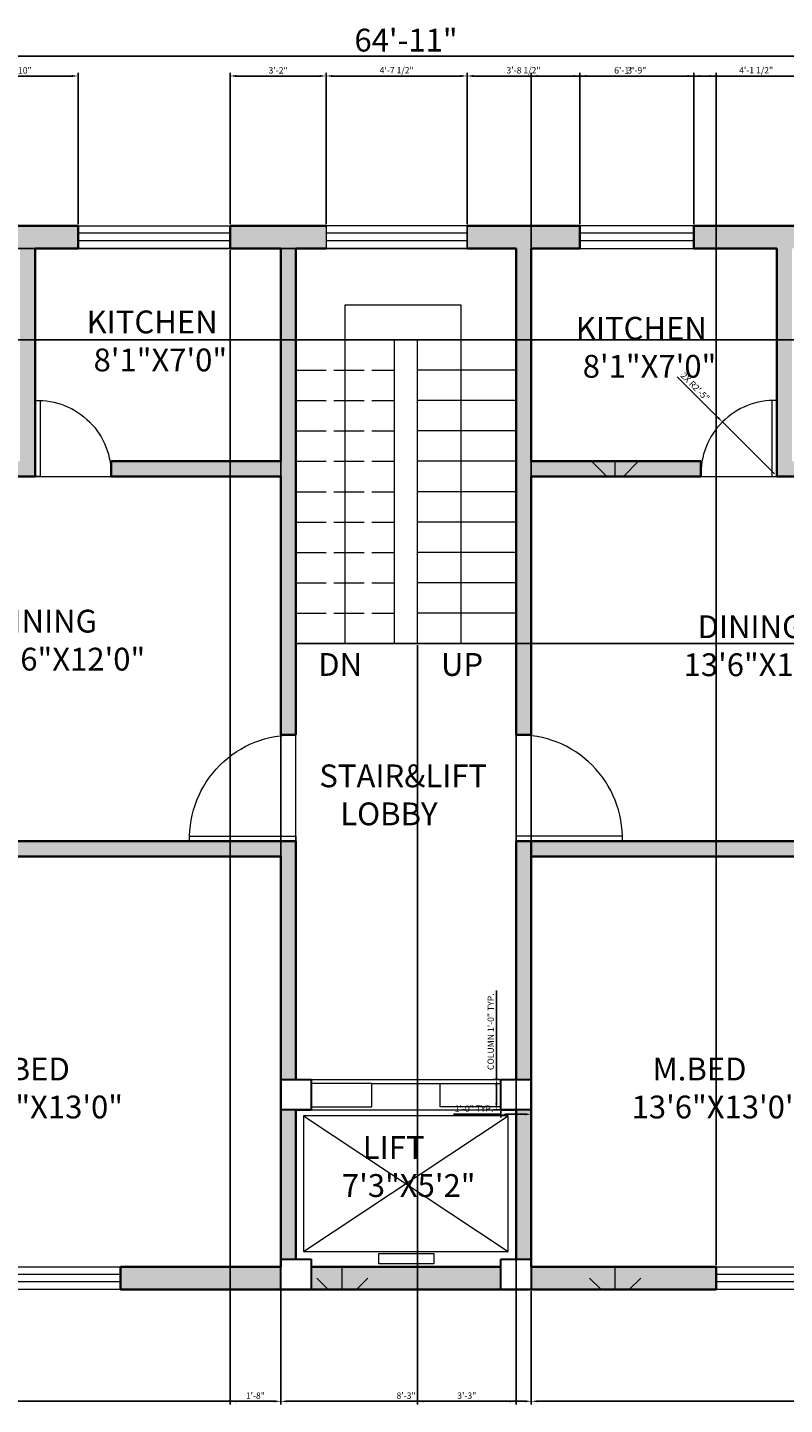
# Model space of a CAD drawing. Units: inches. Extents: x 1851 to 3979, y 3948 to 8145.
# Tile 3 of 4: x 2139 to 2438, y 3948 to 4491. Entities that reach past the tile are written whole.
import ezdxf

# ---------------------------------------------------------------- set-up
doc = ezdxf.new("R2010")
doc.units = ezdxf.units.IN
doc.linetypes.add('ACAD_ISO02W100', pattern=[15, 12, -3])
for name, color, linetype, lineweight in [('A-ANNO-DIMS', 2, 'Continuous', 18), ('A-ANNO-TEXT', 7, 'Continuous', 18), ('A-GLAZ', 140, 'Continuous', 18), ('A-WALL', 7, 'Continuous', 35)]:
    doc.layers.add(name, color=color, linetype=linetype, lineweight=lineweight)
for name, color, linetype, lineweight, true_color in [('A-AREA-IDEN', 9, 'Continuous', 18, 0xc7c8ca), ('A-COLS', 240, 'Continuous', 30, 0xed1f24), ('A-COLS-PATT', 251, 'Continuous', 13, 0x636466), ('A-DOOR', 52, 'Continuous', 18, 0xc8c92d), ('A-FLOR-EVTR', 242, 'Continuous', 18, 0xcd2027), ('A-FLOR-STRS', 242, 'Continuous', 18, 0xcd2027), ('A-FLOR-STRS-OVHD', 242, 'ACAD_ISO02W100', 13, 0xcd2027), ('A-WALL-PATT', 159, 'Continuous', 13, 0x22346e)]:
    doc.layers.add(name, color=color, linetype=linetype, lineweight=lineweight, true_color=true_color)
doc.styles.get("Standard").update_dxf_attribs({"font": 'arial.ttf'})
doc.dimstyles.new('ISO-25', dxfattribs={"dimtxt": 2.5, "dimasz": 2.5, "dimexe": 1.25, "dimexo": 0.625, "dimtad": 1, "dimlunit": 3, "dimtxsty": 'Standard', "dimcen": 2.5, "dimadec": 0, "dimazin": 0, "dimtfac": 1, "dimtmove": 0, "dimatfit": 3, "dimfxl": 1, "dimarcsym": 0})

# ---------------------------------------------------------------- blocks, each defined once
blk = doc.blocks.new('*D1')
at = {"layer": 'A-ANNO-DIMS', "color": 0, "lineweight": -2, "transparency": 16777216}
for p, q in [((1898.74, 4438.02), (1898.74, 4480.98)), ((1901.24, 4479.73), (2675.24, 4479.73)), ((2677.74, 4438.02), (2677.74, 4480.98))]:
    blk.add_line(p, q, dxfattribs=at)
at = {"layer": 'A-ANNO-DIMS', "color": 0, "transparency": 16777216}
for points in [[(1901.24, 4480.15), (1901.24, 4479.31), (1898.74, 4479.73)], [(2675.24, 4480.15), (2675.24, 4479.31), (2677.74, 4479.73)]]:
    blk.add_solid(points, dxfattribs=at)
at = {"layer": 'Defpoints', "color": 0, "transparency": 16777216}
for p in [(2677.74, 4479.73), (1898.74, 4437.39), (2677.74, 4437.39)]:
    blk.add_point(p, dxfattribs=at)
at = {"layer": 'A-ANNO-DIMS', "color": 0, "transparency": 16777216, "insert": (2288.24, 4484.95), "char_height": 9, "attachment_point": 5}
blk.add_mtext('64\'-11"', dxfattribs=at)
blk = doc.blocks.new('DOOR-SINGLE-42IN')
for p, q in [((42, 42), (40, 42)), ((40, 42), (40, 0)), ((42, 0), (42, 42)), ((40, 0), (42, 0))]:
    blk.add_line(p, q)
blk.add_arc((41, 1), 41.01, 88.6028, 181.3972)
blk = doc.blocks.new('DOOR-SINGLE-30IN')
for p, q in [((30, 2), (0, 2)), ((0, 2), (0, 0)), ((0, 0), (30, 0)), ((30, 0), (30, 2))]:
    blk.add_line(p, q)
blk.add_arc((1, 1), 29.02, 358.0251, 91.9749)
blk = doc.blocks.new('WINDOW-60IN')
for p, q in [((0, 9), (60, 9)), ((0, 0), (0, 9)), ((0, 6), (60, 6)), ((60, 9), (60, 0)), ((0, 3), (60, 3)), ((60, 0), (0, 0))]:
    blk.add_line(p, q)
blk = doc.blocks.new('COLUMN-12X12IN')
for p, q in [((0, 0), (0, 12)), ((0, 12), (12, 12)), ((12, 12), (12, 0)), ((12, 0), (0, 0))]:
    blk.add_line(p, q)
blk = doc.blocks.new('*D16')
at = {"layer": 'A-ANNO-DIMS', "color": 0, "lineweight": -2, "transparency": 16777216}
for p, q in [((2323.94, 4075.85), (2323.94, 4110.92)), ((2325.11, 4075.85), (2322.69, 4075.85)), ((2323.94, 4066.35), (2323.94, 4073.35)), ((2325.11, 4063.85), (2322.69, 4063.85))]:
    blk.add_line(p, q, dxfattribs=at)
at = {"layer": 'A-ANNO-DIMS', "color": 0, "transparency": 16777216}
for points in [[(2323.52, 4073.35), (2324.35, 4073.35), (2323.94, 4075.85)], [(2323.52, 4066.35), (2324.35, 4066.35), (2323.94, 4063.85)]]:
    blk.add_solid(points, dxfattribs=at)
at = {"layer": 'Defpoints', "color": 0, "transparency": 16777216}
for p in [(2323.94, 4075.85), (2325.74, 4075.85), (2325.74, 4063.85)]:
    blk.add_point(p, dxfattribs=at)
at = {"layer": 'A-ANNO-DIMS', "color": 0, "transparency": 16777216, "insert": (2322.02, 4094.64), "char_height": 2.5, "attachment_point": 5, "rotation": 90}
blk.add_mtext('COLUMN 1\'-0" TYP.', dxfattribs=at)
blk = doc.blocks.new('*D17')
at = {"layer": 'A-ANNO-DIMS', "color": 0, "lineweight": -2, "transparency": 16777216}
for p, q in [((2325.74, 4062.05), (2306.98, 4062.05)), ((2325.74, 4063.23), (2325.74, 4060.8)), ((2335.24, 4062.05), (2328.24, 4062.05)), ((2337.74, 4063.23), (2337.74, 4060.8))]:
    blk.add_line(p, q, dxfattribs=at)
at = {"layer": 'A-ANNO-DIMS', "color": 0, "transparency": 16777216}
for points in [[(2328.24, 4062.47), (2328.24, 4061.64), (2325.74, 4062.05)], [(2335.24, 4062.47), (2335.24, 4061.64), (2337.74, 4062.05)]]:
    blk.add_solid(points, dxfattribs=at)
at = {"layer": 'Defpoints', "color": 0, "transparency": 16777216}
for p in [(2325.74, 4063.85), (2325.74, 4062.05), (2337.74, 4063.85)]:
    blk.add_point(p, dxfattribs=at)
at = {"layer": 'A-ANNO-DIMS', "color": 0, "transparency": 16777216, "insert": (2315.11, 4063.96), "char_height": 2.5, "attachment_point": 5}
blk.add_mtext('1\'-0" TYP.', dxfattribs=at)
blk = doc.blocks.new('*D24')
at = {"layer": 'A-ANNO-DIMS', "color": 0, "lineweight": -2, "transparency": 16777216}
for p, q in [((1898.74, 3992.23), (1898.74, 3947.5)), ((2238.74, 3992.23), (2238.74, 3947.5)), ((1901.24, 3948.75), (2236.24, 3948.75))]:
    blk.add_line(p, q, dxfattribs=at)
at = {"layer": 'A-ANNO-DIMS', "color": 0, "transparency": 16777216}
for points in [[(1901.24, 3949.17), (1901.24, 3948.34), (1898.74, 3948.75)], [(2236.24, 3949.17), (2236.24, 3948.34), (2238.74, 3948.75)]]:
    blk.add_solid(points, dxfattribs=at)
at = {"layer": 'Defpoints', "color": 0, "transparency": 16777216}
for p in [(1898.74, 3992.85), (2238.74, 3992.85), (2238.74, 3948.75)]:
    blk.add_point(p, dxfattribs=at)
at = {"layer": 'A-ANNO-DIMS', "color": 0, "transparency": 16777216, "insert": (2068.74, 3950.66), "char_height": 2.5, "attachment_point": 5}
blk.add_mtext('28\'-4"', dxfattribs=at)
blk = doc.blocks.new('*D25')
at = {"layer": 'A-ANNO-DIMS', "color": 0, "lineweight": -2, "transparency": 16777216}
for p, q in [((2238.74, 3992.23), (2238.74, 3947.5)), ((2337.74, 3992.23), (2337.74, 3947.5)), ((2241.24, 3948.75), (2335.24, 3948.75))]:
    blk.add_line(p, q, dxfattribs=at)
at = {"layer": 'A-ANNO-DIMS', "color": 0, "transparency": 16777216}
for points in [[(2241.24, 3949.17), (2241.24, 3948.34), (2238.74, 3948.75)], [(2335.24, 3949.17), (2335.24, 3948.34), (2337.74, 3948.75)]]:
    blk.add_solid(points, dxfattribs=at)
at = {"layer": 'Defpoints', "color": 0, "transparency": 16777216}
for p in [(2238.74, 3992.85), (2337.74, 3992.85), (2337.74, 3948.75)]:
    blk.add_point(p, dxfattribs=at)
at = {"layer": 'A-ANNO-DIMS', "color": 0, "transparency": 16777216, "insert": (2288.24, 3950.66), "char_height": 2.5, "attachment_point": 5}
blk.add_mtext('8\'-3"', dxfattribs=at)
blk = doc.blocks.new('*D26')
at = {"layer": 'A-ANNO-DIMS', "color": 0, "lineweight": -2, "transparency": 16777216}
for p, q in [((2337.74, 3992.23), (2337.74, 3947.5)), ((2677.74, 3992.23), (2677.74, 3947.5)), ((2340.24, 3948.75), (2675.24, 3948.75))]:
    blk.add_line(p, q, dxfattribs=at)
at = {"layer": 'A-ANNO-DIMS', "color": 0, "transparency": 16777216}
for points in [[(2340.24, 3949.17), (2340.24, 3948.34), (2337.74, 3948.75)], [(2675.24, 3949.17), (2675.24, 3948.34), (2677.74, 3948.75)]]:
    blk.add_solid(points, dxfattribs=at)
at = {"layer": 'Defpoints', "color": 0, "transparency": 16777216}
for p in [(2337.74, 3992.85), (2677.74, 3992.85), (2677.74, 3948.75)]:
    blk.add_point(p, dxfattribs=at)
at = {"layer": 'A-ANNO-DIMS', "color": 0, "transparency": 16777216, "insert": (2507.74, 3950.66), "char_height": 2.5, "attachment_point": 5}
blk.add_mtext('28\'-4"', dxfattribs=at)
blk = doc.blocks.new('*D29')
at = {"layer": 'A-ANNO-DIMS', "color": 0, "lineweight": -2, "transparency": 16777216}
for p, q in [((2337.74, 4002.48), (2337.74, 4473.2)), ((2340.24, 4471.95), (2408.24, 4471.95)), ((2410.74, 4002.48), (2410.74, 4473.2))]:
    blk.add_line(p, q, dxfattribs=at)
at = {"layer": 'A-ANNO-DIMS', "color": 0, "transparency": 16777216}
for points in [[(2340.24, 4472.37), (2340.24, 4471.54), (2337.74, 4471.95)], [(2408.24, 4472.37), (2408.24, 4471.54), (2410.74, 4471.95)]]:
    blk.add_solid(points, dxfattribs=at)
at = {"layer": 'Defpoints', "color": 0, "transparency": 16777216}
for p in [(2410.74, 4471.95), (2337.74, 4001.85), (2410.74, 4001.85)]:
    blk.add_point(p, dxfattribs=at)
at = {"layer": 'A-ANNO-DIMS', "color": 0, "transparency": 16777216, "insert": (2374.24, 4473.86), "char_height": 2.5, "attachment_point": 5}
blk.add_mtext('6\'-1"', dxfattribs=at)
blk = doc.blocks.new('*D33')
at = {"layer": 'A-ANNO-DIMS', "color": 0, "lineweight": -2, "transparency": 16777216}
for p, q in [((2245.36, 4367.85), (2723.09, 4367.85)), ((2721.84, 4250.35), (2721.84, 4365.35)), ((2245.36, 4247.85), (2723.09, 4247.85))]:
    blk.add_line(p, q, dxfattribs=at)
at = {"layer": 'A-ANNO-DIMS', "color": 0, "transparency": 16777216}
for points in [[(2721.42, 4365.35), (2722.25, 4365.35), (2721.84, 4367.85)], [(2721.42, 4250.35), (2722.25, 4250.35), (2721.84, 4247.85)]]:
    blk.add_solid(points, dxfattribs=at)
at = {"layer": 'Defpoints', "color": 0, "transparency": 16777216}
for p in [(2244.74, 4367.85), (2721.84, 4367.85), (2244.74, 4247.85)]:
    blk.add_point(p, dxfattribs=at)
at = {"layer": 'A-ANNO-DIMS', "color": 0, "transparency": 16777216, "insert": (2719.93, 4307.85), "char_height": 2.5, "attachment_point": 5, "rotation": 90}
blk.add_mtext('10\'-0"', dxfattribs=at)
blk = doc.blocks.new('*D34')
at = {"layer": 'A-ANNO-DIMS', "color": 0, "lineweight": -2, "transparency": 16777216}
for p, q in [((2292.74, 4247.23), (2292.74, 3947.5)), ((2331.74, 4247.23), (2331.74, 3947.5)), ((2295.24, 3948.75), (2329.24, 3948.75))]:
    blk.add_line(p, q, dxfattribs=at)
at = {"layer": 'A-ANNO-DIMS', "color": 0, "transparency": 16777216}
for points in [[(2295.24, 3949.17), (2295.24, 3948.34), (2292.74, 3948.75)], [(2329.24, 3949.17), (2329.24, 3948.34), (2331.74, 3948.75)]]:
    blk.add_solid(points, dxfattribs=at)
at = {"layer": 'Defpoints', "color": 0, "transparency": 16777216}
for p in [(2292.74, 4247.85), (2331.74, 4247.85), (2331.74, 3948.75)]:
    blk.add_point(p, dxfattribs=at)
at = {"layer": 'A-ANNO-DIMS', "color": 0, "transparency": 16777216, "insert": (2312.24, 3950.66), "char_height": 2.5, "attachment_point": 5}
blk.add_mtext('3\'-3"', dxfattribs=at)
blk = doc.blocks.new('*D35')
at = {"layer": 'A-ANNO-DIMS', "color": 0, "lineweight": -2, "transparency": 16777216}
for p, q in [((2331.11, 4403.85), (1853.39, 4403.85)), ((1854.64, 4370.35), (1854.64, 4401.35)), ((2331.11, 4367.85), (1853.39, 4367.85))]:
    blk.add_line(p, q, dxfattribs=at)
at = {"layer": 'A-ANNO-DIMS', "color": 0, "transparency": 16777216}
for points in [[(1854.22, 4401.35), (1855.05, 4401.35), (1854.64, 4403.85)], [(1854.22, 4370.35), (1855.05, 4370.35), (1854.64, 4367.85)]]:
    blk.add_solid(points, dxfattribs=at)
at = {"layer": 'Defpoints', "color": 0, "transparency": 16777216}
for p in [(1854.64, 4403.85), (2331.74, 4403.85), (2331.74, 4367.85)]:
    blk.add_point(p, dxfattribs=at)
at = {"layer": 'A-ANNO-DIMS', "color": 0, "transparency": 16777216, "insert": (1852.73, 4385.85), "char_height": 2.5, "attachment_point": 5, "rotation": 90}
blk.add_mtext('3\'-0"', dxfattribs=at)
blk = doc.blocks.new('*D44')
at = {"layer": 'A-ANNO-DIMS', "color": 0, "lineweight": -2, "transparency": 16777216}
for p, q in [((2256.69, 4413.48), (2256.69, 4473.2)), ((2259.19, 4471.95), (2309.87, 4471.95)), ((2312.37, 4413.48), (2312.37, 4473.2))]:
    blk.add_line(p, q, dxfattribs=at)
at = {"layer": 'A-ANNO-DIMS', "color": 0, "transparency": 16777216}
for points in [[(2259.19, 4472.37), (2259.19, 4471.54), (2256.69, 4471.95)], [(2309.87, 4472.37), (2309.87, 4471.54), (2312.37, 4471.95)]]:
    blk.add_solid(points, dxfattribs=at)
at = {"layer": 'Defpoints', "color": 0, "transparency": 16777216}
for p in [(2312.37, 4471.95), (2256.69, 4412.85), (2312.37, 4412.85)]:
    blk.add_point(p, dxfattribs=at)
at = {"layer": 'A-ANNO-DIMS', "color": 0, "transparency": 16777216, "insert": (2284.53, 4473.87), "char_height": 2.5, "attachment_point": 5}
blk.add_mtext('4\'-7 1/2"', dxfattribs=at)
blk = doc.blocks.new('*D45')
at = {"layer": 'A-ANNO-DIMS', "color": 0, "lineweight": -2, "transparency": 16777216}
for p, q in [((2356.91, 4413.48), (2356.91, 4473.2)), ((2359.41, 4471.95), (2399.38, 4471.95)), ((2401.88, 4413.48), (2401.88, 4473.2))]:
    blk.add_line(p, q, dxfattribs=at)
at = {"layer": 'A-ANNO-DIMS', "color": 0, "transparency": 16777216}
for points in [[(2359.41, 4472.37), (2359.41, 4471.54), (2356.91, 4471.95)], [(2399.38, 4472.37), (2399.38, 4471.54), (2401.88, 4471.95)]]:
    blk.add_solid(points, dxfattribs=at)
at = {"layer": 'Defpoints', "color": 0, "transparency": 16777216}
for p in [(2401.88, 4471.95), (2356.91, 4412.85), (2401.88, 4412.85)]:
    blk.add_point(p, dxfattribs=at)
at = {"layer": 'A-ANNO-DIMS', "color": 0, "transparency": 16777216, "insert": (2379.4, 4473.86), "char_height": 2.5, "attachment_point": 5}
blk.add_mtext('3\'-9"', dxfattribs=at)
blk = doc.blocks.new('*D48')
at = {"layer": 'A-ANNO-DIMS', "color": 0, "lineweight": -2, "transparency": 16777216}
for p, q in [((2218.72, 4403.23), (2218.72, 3947.5)), ((2238.74, 4403.23), (2238.74, 3947.5)), ((2221.22, 3948.75), (2236.24, 3948.75))]:
    blk.add_line(p, q, dxfattribs=at)
at = {"layer": 'A-ANNO-DIMS', "color": 0, "transparency": 16777216}
for points in [[(2221.22, 3949.17), (2221.22, 3948.34), (2218.72, 3948.75)], [(2236.24, 3949.17), (2236.24, 3948.34), (2238.74, 3948.75)]]:
    blk.add_solid(points, dxfattribs=at)
at = {"layer": 'Defpoints', "color": 0, "transparency": 16777216}
for p in [(2218.72, 4403.85), (2238.74, 4403.85), (2238.74, 3948.75)]:
    blk.add_point(p, dxfattribs=at)
at = {"layer": 'A-ANNO-DIMS', "color": 0, "transparency": 16777216, "insert": (2228.73, 3950.66), "char_height": 2.5, "attachment_point": 5}
blk.add_mtext('1\'-8"', dxfattribs=at)
blk = doc.blocks.new('*D49')
at = {"layer": 'A-ANNO-DIMS', "color": 0, "lineweight": -2, "transparency": 16777216}
for p, q in [((2112.59, 4413.48), (2112.59, 4473.2)), ((2115.09, 4471.95), (2156.22, 4471.95)), ((2158.72, 4413.48), (2158.72, 4473.2))]:
    blk.add_line(p, q, dxfattribs=at)
at = {"layer": 'A-ANNO-DIMS', "color": 0, "transparency": 16777216}
for points in [[(2115.09, 4472.37), (2115.09, 4471.54), (2112.59, 4471.95)], [(2156.22, 4472.37), (2156.22, 4471.54), (2158.72, 4471.95)]]:
    blk.add_solid(points, dxfattribs=at)
at = {"layer": 'Defpoints', "color": 0, "transparency": 16777216}
for p in [(2158.72, 4471.95), (2112.59, 4412.85), (2158.72, 4412.85)]:
    blk.add_point(p, dxfattribs=at)
at = {"layer": 'A-ANNO-DIMS', "color": 0, "transparency": 16777216, "insert": (2135.66, 4473.86), "char_height": 2.5, "attachment_point": 5}
blk.add_mtext('3\'-10"', dxfattribs=at)
blk = doc.blocks.new('*D50')
at = {"layer": 'A-ANNO-DIMS', "color": 0, "lineweight": -2, "transparency": 16777216}
for p, q in [((2218.72, 4413.48), (2218.72, 4473.2)), ((2221.22, 4471.95), (2254.19, 4471.95)), ((2256.69, 4413.48), (2256.69, 4473.2))]:
    blk.add_line(p, q, dxfattribs=at)
at = {"layer": 'A-ANNO-DIMS', "color": 0, "transparency": 16777216}
for points in [[(2221.22, 4472.37), (2221.22, 4471.54), (2218.72, 4471.95)], [(2254.19, 4472.37), (2254.19, 4471.54), (2256.69, 4471.95)]]:
    blk.add_solid(points, dxfattribs=at)
at = {"layer": 'Defpoints', "color": 0, "transparency": 16777216}
for p in [(2256.69, 4471.95), (2218.72, 4412.85), (2256.69, 4412.85)]:
    blk.add_point(p, dxfattribs=at)
at = {"layer": 'A-ANNO-DIMS', "color": 0, "transparency": 16777216, "insert": (2237.71, 4473.86), "char_height": 2.5, "attachment_point": 5}
blk.add_mtext('3\'-2"', dxfattribs=at)
blk = doc.blocks.new('*D51')
at = {"layer": 'A-ANNO-DIMS', "color": 0, "lineweight": -2, "transparency": 16777216}
for p, q in [((2312.37, 4413.48), (2312.37, 4473.2)), ((2314.87, 4471.95), (2354.41, 4471.95)), ((2356.91, 4413.48), (2356.91, 4473.2))]:
    blk.add_line(p, q, dxfattribs=at)
at = {"layer": 'A-ANNO-DIMS', "color": 0, "transparency": 16777216}
for points in [[(2314.87, 4472.37), (2314.87, 4471.54), (2312.37, 4471.95)], [(2354.41, 4472.37), (2354.41, 4471.54), (2356.91, 4471.95)]]:
    blk.add_solid(points, dxfattribs=at)
at = {"layer": 'Defpoints', "color": 0, "transparency": 16777216}
for p in [(2356.91, 4471.95), (2312.37, 4412.85), (2356.91, 4412.85)]:
    blk.add_point(p, dxfattribs=at)
at = {"layer": 'A-ANNO-DIMS', "color": 0, "transparency": 16777216, "insert": (2334.64, 4473.87), "char_height": 2.5, "attachment_point": 5}
blk.add_mtext('3\'-8 1/2"', dxfattribs=at)
blk = doc.blocks.new('*D52')
at = {"layer": 'A-ANNO-DIMS', "color": 0, "lineweight": -2, "transparency": 16777216}
for p, q in [((2401.88, 4413.48), (2401.88, 4473.2)), ((2404.38, 4471.95), (2448.67, 4471.95)), ((2451.17, 4413.48), (2451.17, 4473.2))]:
    blk.add_line(p, q, dxfattribs=at)
at = {"layer": 'A-ANNO-DIMS', "color": 0, "transparency": 16777216}
for points in [[(2404.38, 4472.37), (2404.38, 4471.54), (2401.88, 4471.95)], [(2448.67, 4472.37), (2448.67, 4471.54), (2451.17, 4471.95)]]:
    blk.add_solid(points, dxfattribs=at)
at = {"layer": 'Defpoints', "color": 0, "transparency": 16777216}
for p in [(2451.17, 4471.95), (2401.88, 4412.85), (2451.17, 4412.85)]:
    blk.add_point(p, dxfattribs=at)
at = {"layer": 'A-ANNO-DIMS', "color": 0, "transparency": 16777216, "insert": (2426.53, 4473.87), "char_height": 2.5, "attachment_point": 5}
blk.add_mtext('4\'-1 1/2"', dxfattribs=at)
blk = doc.blocks.new('*D55')
at = {"layer": 'A-ANNO-DIMS', "color": 0, "lineweight": -2, "transparency": 16777216}
for p, q in [((2395.36, 4353.24), (2411.45, 4337.14)), ((2433.74, 4314.85), (2413.22, 4335.37))]:
    blk.add_line(p, q, dxfattribs=at)
at = {"layer": 'A-ANNO-DIMS', "color": 0, "transparency": 16777216}
blk.add_solid([(2411.74, 4337.44), (2411.16, 4336.85), (2413.22, 4335.37)], dxfattribs=at)
at = {"layer": 'Defpoints', "color": 0, "transparency": 16777216}
for p in [(2413.22, 4335.37), (2433.74, 4314.85)]:
    blk.add_point(p, dxfattribs=at)
at = {"layer": 'A-ANNO-DIMS', "color": 0, "transparency": 16777216, "insert": (2402.25, 4349.03), "char_height": 2.5, "attachment_point": 5, "rotation": 315}
blk.add_mtext('2X R2\'-5"', dxfattribs=at)

msp = doc.modelspace()

# ---------------------------------------------------------------- hatches: boundary and pattern name
at = {"layer": 'A-COLS-PATT'}
h = msp.add_hatch(dxfattribs=at)
h.set_pattern_fill('GRASS', color=256, scale=3)
h.paths.add_polyline_path([(2250.736, 4004.855), (2238.736, 4004.855), (2238.736, 3992.855), (2250.736, 3992.855)])
h.paths.add_polyline_path([(2250.736, 4075.855), (2238.736, 4075.855), (2238.736, 4063.855), (2250.736, 4063.855)])
h.paths.add_polyline_path([(2337.736, 4075.855), (2325.736, 4075.855), (2325.736, 4063.855), (2337.736, 4063.855)])
h.paths.add_polyline_path([(2337.736, 4004.855), (2325.736, 4004.855), (2325.736, 3992.855), (2337.736, 3992.855)])
at = {"layer": 'A-WALL-PATT'}
h = msp.add_hatch(dxfattribs=at)
h.set_pattern_fill('GRASS', color=256, scale=3)
h.paths.add_polyline_path([(1942.655, 4412.855), (1898.736, 4412.855), (1898.736, 4348.625), (1907.736, 4348.625), (1907.736, 4403.855), (1942.655, 4403.855)])
h.paths.add_polyline_path([(2027.97, 4412.855), (2002.655, 4412.855), (2002.655, 4403.855), (2027.97, 4403.855, -0.0293864), (2027.97, 4405.855)])
h.paths.add_polyline_path([(2088.59, 4412.855), (2045.97, 4412.855), (2045.97, 4403.855), (2069.736, 4403.855), (2069.736, 4349.855, -0.0172363), (2071.736, 4349.855), (2075.736, 4349.855), (2075.736, 4403.855), (2088.59, 4403.855)])
h.paths.add_polyline_path([(2158.724, 4412.855), (2112.59, 4412.855), (2112.59, 4403.855), (2135.736, 4403.855), (2135.736, 4319.855), (2069.736, 4319.855), (2069.736, 4241.855), (2075.736, 4241.855), (2075.736, 4313.855), (2141.736, 4313.855), (2141.736, 4403.855), (2158.724, 4403.855)])
h.paths.add_polyline_path([(2244.736, 4403.855), (2256.687, 4403.855), (2256.687, 4412.855), (2218.724, 4412.855), (2218.724, 4403.855), (2238.736, 4403.855), (2238.736, 4319.855), (2171.736, 4319.855), (2171.736, 4315.855, -0.0172363), (2171.736, 4313.855), (2238.736, 4313.855), (2238.736, 4211.855), (2242.736, 4211.855, -0.0121933), (2244.736, 4211.855)])
h.paths.add_polyline_path([(2356.912, 4412.855), (2353.884, 4412.855), (2312.372, 4412.855), (2312.372, 4403.855), (2331.736, 4403.855), (2331.736, 4211.855, -0.0121933), (2333.736, 4211.855), (2337.736, 4211.855), (2337.736, 4313.855), (2404.736, 4313.855, -0.0172363), (2404.736, 4315.855), (2404.736, 4319.855), (2337.736, 4319.855), (2337.736, 4403.855), (2353.884, 4403.855), (2356.912, 4403.855)])
h.paths.add_polyline_path([(2440.736, 4403.855), (2451.168, 4403.855), (2451.168, 4412.855), (2401.884, 4412.855), (2401.884, 4403.855), (2434.736, 4403.855), (2434.736, 4313.855), (2500.736, 4313.855), (2500.736, 4241.855), (2506.736, 4241.855), (2506.736, 4283.855), (2506.736, 4319.855), (2476.736, 4319.855), (2440.736, 4319.855)])
h.paths.add_polyline_path([(2506.736, 4403.855), (2516.983, 4403.855), (2516.983, 4412.855), (2475.168, 4412.855), (2475.168, 4403.855), (2500.736, 4403.855), (2500.736, 4349.855), (2504.736, 4349.855, -0.0172363), (2506.736, 4349.855)])
h.paths.add_polyline_path([(2544.739, 4412.855), (2534.983, 4412.855), (2534.983, 4405.855, -0.0293864), (2534.983, 4403.855), (2544.739, 4403.855)])
h.paths.add_polyline_path([(2677.736, 4412.855), (2618.736, 4412.855), (2616.739, 4412.855), (2616.739, 4403.855), (2668.736, 4403.855), (2668.736, 4349.414), (2677.736, 4349.414), (2677.736, 4403.855)])
h.paths.add_polyline_path([(2677.736, 4301.414), (2668.736, 4301.414), (2668.736, 4247.855), (2548.736, 4247.855), (2548.736, 4243.855, -0.0121933), (2548.736, 4241.855), (2572.736, 4241.855), (2572.736, 4187.855, -0.0293864), (2574.736, 4187.855), (2578.736, 4187.855), (2578.736, 4241.855), (2668.736, 4241.855), (2668.736, 4216.247), (2677.736, 4216.247)])
h.paths.add_polyline_path([(2677.736, 4192.247), (2668.736, 4192.247), (2668.736, 4169.855), (2572.736, 4169.855), (2548.736, 4169.855, -0.0424267), (2549.319, 4163.855), (2572.736, 4163.855), (2668.736, 4163.855), (2668.736, 4130.251), (2677.736, 4130.251)])
h.paths.add_polyline_path([(2677.736, 4001.855), (2677.736, 4058.251), (2668.736, 4058.251), (2668.736, 4001.855), (2614.828, 4001.855), (2614.828, 3992.855), (2618.736, 3992.855), (2677.736, 3992.855)])
h.paths.add_polyline_path([(2554.828, 4001.855), (2512.736, 4001.855), (2512.736, 4163.855), (2512.736, 4169.855), (2506.736, 4169.855), (2506.736, 4127.855), (2506.736, 4001.855), (2470.736, 4001.855), (2470.736, 3992.855), (2554.828, 3992.855)])
h.paths.add_polyline_path([(2410.736, 4001.855), (2337.736, 4001.855), (2337.736, 3992.855), (2410.736, 3992.855)])
h.paths.add_polyline_path([(2337.736, 4169.855), (2331.736, 4169.855), (2331.736, 4075.855), (2337.736, 4075.855)])
h.paths.add_polyline_path([(2464.736, 4167.855, -0.0121933), (2464.736, 4169.855), (2337.736, 4169.855), (2337.736, 4163.855), (2464.736, 4163.855)])
h.paths.add_polyline_path([(2244.736, 4169.855), (2202.736, 4169.855), (2117.736, 4169.855, -0.0121933), (2117.736, 4167.855), (2117.736, 4163.855), (2238.736, 4163.855), (2238.736, 4075.855), (2244.736, 4075.855)])
h.paths.add_polyline_path([(2325.736, 4001.855), (2250.736, 4001.855), (2250.736, 3992.855), (2325.736, 3992.855)])
h.paths.add_polyline_path([(2238.736, 4001.855), (2175.511, 4001.855), (2175.511, 3992.855), (2238.736, 3992.855)])
h.paths.add_polyline_path([(2115.511, 4001.855), (2075.736, 4001.855), (2075.736, 4169.855), (2069.736, 4169.855), (2069.736, 4127.855), (2069.736, 4001.855), (2009.539, 4001.855), (2009.539, 3992.855), (2115.511, 3992.855)])
h.paths.add_polyline_path([(1949.539, 4001.855), (1907.736, 4001.855), (1907.736, 4049.088), (1898.736, 4049.088), (1898.736, 3992.855), (1949.539, 3992.855)])
h.paths.add_polyline_path([(1907.736, 4163.855), (2027.736, 4163.855), (2027.736, 4167.855, -0.0121933), (2027.736, 4169.855), (1907.736, 4169.855), (1907.736, 4195.575), (1898.736, 4195.575), (1898.736, 4109.088), (1907.736, 4109.088)])
h.paths.add_polyline_path([(2027.736, 4247.855), (1907.736, 4247.855), (1907.736, 4288.625), (1898.736, 4288.625), (1898.736, 4219.575), (1907.736, 4219.575), (1907.736, 4241.855), (2003.736, 4241.855), (2003.736, 4219.575), (2003.736, 4199.855), (2007.736, 4199.855, -0.0172363), (2009.736, 4199.855), (2009.736, 4241.855), (2027.736, 4241.855, -0.0121933), (2027.736, 4243.855)])
h = msp.add_hatch(dxfattribs=at)
h.set_pattern_fill('GRASS', color=256, scale=3)
h.paths.add_polyline_path([(1942.655, 4412.855), (1898.736, 4412.855), (1898.736, 4348.625), (1907.736, 4348.625), (1907.736, 4403.855), (1942.655, 4403.855)])
h.paths.add_polyline_path([(2027.97, 4412.855), (2002.655, 4412.855), (2002.655, 4403.855), (2027.97, 4403.855, -0.0293864), (2027.97, 4405.855)])
h.paths.add_polyline_path([(2088.59, 4412.855), (2045.97, 4412.855), (2045.97, 4403.855), (2069.736, 4403.855), (2069.736, 4349.855, -0.0172363), (2071.736, 4349.855), (2075.736, 4349.855), (2075.736, 4403.855), (2088.59, 4403.855)])
h.paths.add_polyline_path([(2158.724, 4412.855), (2112.59, 4412.855), (2112.59, 4403.855), (2135.736, 4403.855), (2135.736, 4319.855), (2069.736, 4319.855), (2069.736, 4241.855), (2075.736, 4241.855), (2075.736, 4313.855), (2141.736, 4313.855), (2141.736, 4343.855), (2141.736, 4403.855), (2158.724, 4403.855)])
h.paths.add_polyline_path([(2256.687, 4412.855), (2218.724, 4412.855), (2218.724, 4403.855), (2238.736, 4403.855), (2238.736, 4319.855), (2171.736, 4319.855), (2171.736, 4315.855, -0.0172363), (2171.736, 4313.855), (2238.736, 4313.855), (2238.736, 4211.855), (2242.736, 4211.855, -0.0121933), (2244.736, 4211.855), (2244.736, 4403.855), (2256.687, 4403.855)])
h.paths.add_polyline_path([(2356.912, 4412.855), (2353.884, 4412.855), (2312.372, 4412.855), (2312.372, 4403.855), (2331.736, 4403.855), (2331.736, 4211.855, -0.0121933), (2333.736, 4211.855), (2337.736, 4211.855), (2337.736, 4313.855), (2404.736, 4313.855, -0.0172363), (2404.736, 4315.855), (2404.736, 4319.855), (2337.736, 4319.855), (2337.736, 4403.855), (2353.884, 4403.855), (2356.912, 4403.855)])
h = msp.add_hatch(color=256, dxfattribs=at)
h.dxf.hatch_style = 1
h.paths.add_polyline_path([(1907.736, 4163.855), (2027.736, 4163.855), (2027.736, 4167.855, -0.0121933), (2027.736, 4169.855), (1907.736, 4169.855), (1907.736, 4195.575), (1898.736, 4195.575), (1898.736, 4109.088), (1907.736, 4109.088)])
h.paths.add_polyline_path([(1907.736, 4049.088), (1898.736, 4049.088), (1898.736, 3992.855), (1949.539, 3992.855), (1949.539, 4001.855), (1907.736, 4001.855)])
h.paths.add_polyline_path([(2115.511, 4001.855), (2075.736, 4001.855), (2075.736, 4169.855), (2069.736, 4169.855), (2069.736, 4127.855), (2069.736, 4001.855), (2009.539, 4001.855), (2009.539, 3992.855), (2115.511, 3992.855)])
h.paths.add_polyline_path([(2238.736, 4001.855), (2175.511, 4001.855), (2175.511, 3992.855), (2238.736, 3992.855)])
h.paths.add_polyline_path([(2325.736, 4001.855), (2250.736, 4001.855), (2250.736, 3992.855), (2325.736, 3992.855)])
h.paths.add_polyline_path([(2410.736, 4001.855), (2337.736, 4001.855), (2337.736, 3992.855), (2410.736, 3992.855)])
h.paths.add_polyline_path([(2554.828, 4001.855), (2512.736, 4001.855), (2512.736, 4163.855), (2512.736, 4169.855), (2506.736, 4169.855), (2506.736, 4127.855), (2506.736, 4001.855), (2470.736, 4001.855), (2470.736, 3992.855), (2554.828, 3992.855)])
h.paths.add_polyline_path([(2677.736, 4001.855), (2677.736, 4058.251), (2668.736, 4058.251), (2668.736, 4001.855), (2614.828, 4001.855), (2614.828, 3992.855), (2618.736, 3992.855), (2677.736, 3992.855)])
h.paths.add_polyline_path([(2244.736, 4169.855), (2202.736, 4169.855), (2117.736, 4169.855, -0.0121933), (2117.736, 4167.855), (2117.736, 4163.855), (2238.736, 4163.855), (2238.736, 4075.855), (2244.736, 4075.855)])
h.paths.add_polyline_path([(2337.736, 4169.855), (2331.736, 4169.855), (2331.736, 4075.855), (2337.736, 4075.855)])
h.paths.add_polyline_path([(2337.736, 4063.855), (2331.736, 4063.855), (2331.736, 4004.855), (2337.736, 4004.855)])
h.paths.add_polyline_path([(2244.736, 4063.855), (2238.736, 4063.855), (2238.736, 4004.855), (2244.736, 4004.855)])
h.paths.add_polyline_path([(2464.736, 4167.855, -0.0121933), (2464.736, 4169.855), (2337.736, 4169.855), (2337.736, 4163.855), (2464.736, 4163.855)])
h.paths.add_polyline_path([(2337.736, 4313.855), (2404.736, 4313.855, -0.0172363), (2404.736, 4315.855), (2404.736, 4319.855), (2337.736, 4319.855), (2337.736, 4403.855), (2353.884, 4403.855), (2356.912, 4403.855), (2356.912, 4412.855), (2353.884, 4412.855), (2312.372, 4412.855), (2312.372, 4403.855), (2331.736, 4403.855), (2331.736, 4211.855, -0.0121933), (2333.736, 4211.855), (2337.736, 4211.855)])
h.paths.add_polyline_path([(2244.736, 4403.855), (2256.687, 4403.855), (2256.687, 4412.855), (2218.724, 4412.855), (2218.724, 4403.855), (2238.736, 4403.855), (2238.736, 4319.855), (2171.736, 4319.855), (2171.736, 4315.855, -0.0172363), (2171.736, 4313.855), (2238.736, 4313.855), (2238.736, 4211.855), (2242.736, 4211.855, -0.0121933), (2244.736, 4211.855)])
h.paths.add_polyline_path([(2506.736, 4283.855), (2506.736, 4319.855), (2476.736, 4319.855), (2440.736, 4319.855), (2440.736, 4403.855), (2451.168, 4403.855), (2451.168, 4412.855), (2401.884, 4412.855), (2401.884, 4403.855), (2434.736, 4403.855), (2434.736, 4313.855), (2500.736, 4313.855), (2500.736, 4241.855), (2506.736, 4241.855)])
h.paths.add_polyline_path([(2578.736, 4241.855), (2668.736, 4241.855), (2668.736, 4216.247), (2677.736, 4216.247), (2677.736, 4301.414), (2668.736, 4301.414), (2668.736, 4247.855), (2548.736, 4247.855), (2548.736, 4243.855, -0.0121933), (2548.736, 4241.855), (2572.736, 4241.855), (2572.736, 4187.855, -0.0293864), (2574.736, 4187.855), (2578.736, 4187.855)])
h.paths.add_polyline_path([(2677.736, 4192.247), (2668.736, 4192.247), (2668.736, 4169.855), (2572.736, 4169.855), (2548.736, 4169.855, -0.0424267), (2549.319, 4163.855), (2572.736, 4163.855), (2668.736, 4163.855), (2668.736, 4130.251), (2677.736, 4130.251)])
h.paths.add_polyline_path([(2506.736, 4403.855), (2516.983, 4403.855), (2516.983, 4412.855), (2475.168, 4412.855), (2475.168, 4403.855), (2500.736, 4403.855), (2500.736, 4349.855), (2504.736, 4349.855, -0.0172363), (2506.736, 4349.855)])
h.paths.add_polyline_path([(2677.736, 4412.855), (2618.736, 4412.855), (2616.739, 4412.855), (2616.739, 4403.855), (2668.736, 4403.855), (2668.736, 4349.414), (2677.736, 4349.414), (2677.736, 4403.855)])
h.paths.add_polyline_path([(2544.739, 4412.855), (2534.983, 4412.855), (2534.983, 4405.855, -0.0293864), (2534.983, 4403.855), (2544.739, 4403.855)])
h.paths.add_polyline_path([(2141.736, 4403.855), (2158.724, 4403.855), (2158.724, 4412.855), (2112.59, 4412.855), (2112.59, 4403.855), (2135.736, 4403.855), (2135.736, 4319.855), (2069.736, 4319.855), (2069.736, 4241.855), (2075.736, 4241.855), (2075.736, 4313.855), (2141.736, 4313.855), (2141.736, 4343.855)])
h.paths.add_polyline_path([(2075.736, 4403.855), (2088.59, 4403.855), (2088.59, 4412.855), (2045.97, 4412.855), (2045.97, 4403.855), (2069.736, 4403.855), (2069.736, 4349.855, -0.0172363), (2071.736, 4349.855), (2075.736, 4349.855)])
h.paths.add_polyline_path([(2027.97, 4412.855), (2002.655, 4412.855), (2002.655, 4403.855), (2027.97, 4403.855, -0.0293864), (2027.97, 4405.855)])
h.paths.add_polyline_path([(1942.655, 4412.855), (1898.736, 4412.855), (1898.736, 4348.625), (1907.736, 4348.625), (1907.736, 4403.855), (1942.655, 4403.855)])
h.paths.add_polyline_path([(2027.736, 4247.855), (1907.736, 4247.855), (1907.736, 4288.625), (1898.736, 4288.625), (1898.736, 4219.575), (1907.736, 4219.575), (1907.736, 4241.855), (2003.736, 4241.855), (2003.736, 4219.575), (2003.736, 4199.855), (2007.736, 4199.855, -0.0172363), (2009.736, 4199.855), (2009.736, 4241.855), (2027.736, 4241.855, -0.0121933), (2027.736, 4243.855)])

# ---------------------------------------------------------------- linework, layer by layer
at = {"layer": 'A-DOOR'}
for p, q in [((2141.736, 4313.855), (2171.736, 4313.855)), ((2404.736, 4313.855), (2434.736, 4313.855)), ((2244.736, 4169.855), (2244.736, 4211.855)), ((2331.736, 4169.855), (2331.736, 4211.855))]:
    msp.add_line(p, q, dxfattribs=at)
at = {"layer": 'A-FLOR-EVTR'}
for p, q in [((2250.736, 4075.855), (2325.736, 4075.855)), ((2274.736, 4074.149), (2250.736, 4074.149)), ((2274.736, 4065.067), (2274.736, 4074.149)), ((2274.736, 4074.149), (2301.736, 4074.149)), ((2301.736, 4065.067), (2301.736, 4074.149)), ((2301.736, 4074.149), (2325.736, 4074.149)), ((2247.736, 4061.471), (2247.736, 4007.931)), ((2328.606, 4061.471), (2247.736, 4061.471)), ((2247.736, 4007.931), (2328.606, 4061.471)), ((2247.736, 4061.471), (2328.606, 4007.931)), ((2250.736, 4065.067), (2274.736, 4065.067)), ((2250.736, 4063.855), (2325.736, 4063.855)), ((2325.736, 4065.067), (2301.736, 4065.067)), ((2328.606, 4007.931), (2328.606, 4061.471)), ((2247.736, 4007.931), (2328.606, 4007.931))]:
    msp.add_line(p, q, dxfattribs=at)
msp.add_lwpolyline([(2277.494, 4007.098), (2299.19, 4007.098), (2299.19, 4002.997), (2277.494, 4002.997)], close=True, dxfattribs=at)
at = {"layer": 'A-FLOR-STRS'}
for p, q in [((2264.236, 4247.855), (2264.236, 4381.568)), ((2264.236, 4381.568), (2309.947, 4381.568)), ((2309.947, 4381.568), (2309.947, 4247.855)), ((2283.736, 4367.855), (2331.736, 4367.855)), ((2331.736, 4367.855), (2283.736, 4367.855)), ((2283.736, 4247.855), (2283.736, 4367.855)), ((2292.736, 4247.855), (2292.736, 4367.855)), ((2331.736, 4355.855), (2292.736, 4355.855)), ((2331.736, 4343.855), (2292.736, 4343.855)), ((2331.736, 4331.855), (2292.736, 4331.855)), ((2331.736, 4319.855), (2292.736, 4319.855)), ((2331.736, 4307.855), (2292.736, 4307.855)), ((2331.736, 4295.855), (2292.736, 4295.855)), ((2331.736, 4283.855), (2292.736, 4283.855)), ((2331.736, 4271.855), (2292.736, 4271.855)), ((2331.736, 4259.855), (2292.736, 4259.855)), ((2283.736, 4247.855), (2264.236, 4247.855)), ((2331.736, 4247.855), (2283.736, 4247.855))]:
    msp.add_line(p, q, dxfattribs=at)
at = {"layer": 'A-FLOR-STRS-OVHD'}
for p, q in [((2244.736, 4367.855), (2283.736, 4367.855)), ((2244.736, 4355.855), (2283.736, 4355.855)), ((2244.736, 4343.855), (2283.736, 4343.855)), ((2244.736, 4331.855), (2283.736, 4331.855)), ((2244.736, 4319.855), (2283.736, 4319.855)), ((2244.736, 4307.855), (2283.736, 4307.855)), ((2244.736, 4295.855), (2283.736, 4295.855)), ((2244.736, 4283.855), (2283.736, 4283.855)), ((2244.736, 4283.855), (2283.736, 4283.855)), ((2244.736, 4271.855), (2283.736, 4271.855)), ((2244.736, 4259.855), (2283.736, 4259.855)), ((2244.736, 4247.855), (2283.736, 4247.855))]:
    msp.add_line(p, q, dxfattribs=at)
at = {"layer": 'A-GLAZ'}
for p, q in [((2256.687, 4412.855), (2256.687, 4403.855)), ((2312.372, 4412.855), (2256.687, 4412.855)), ((2312.372, 4409.855), (2256.687, 4409.855)), ((2312.372, 4412.855), (2312.372, 4403.855)), ((2312.372, 4403.855), (2312.372, 4412.855)), ((2356.912, 4412.855), (2356.912, 4403.855)), ((2401.884, 4412.855), (2356.912, 4412.855)), ((2401.884, 4409.855), (2356.912, 4409.855)), ((2401.884, 4403.855), (2401.884, 4412.855)), ((2312.372, 4406.855), (2256.687, 4406.855)), ((2256.687, 4403.855), (2312.372, 4403.855)), ((2401.884, 4406.855), (2356.912, 4406.855)), ((2356.912, 4403.855), (2401.884, 4403.855))]:
    msp.add_line(p, q, dxfattribs=at)
at = {"layer": 'A-WALL'}
for p, q in [((2112.59, 4412.855), (2158.724, 4412.855)), ((2158.724, 4412.855), (2158.724, 4403.855)), ((2218.724, 4412.855), (2218.724, 4403.855)), ((2218.724, 4412.855), (2256.687, 4412.855)), ((2312.372, 4412.855), (2353.884, 4412.855)), ((2353.884, 4412.855), (2356.912, 4412.855)), ((2356.912, 4412.855), (2356.912, 4403.855)), ((2401.884, 4412.855), (2401.884, 4403.855)), ((2401.884, 4412.855), (2451.168, 4412.855)), ((2141.736, 4313.855), (2141.736, 4403.855)), ((2141.736, 4403.855), (2158.724, 4403.855)), ((2218.724, 4403.855), (2238.736, 4403.855)), ((2238.736, 4319.855), (2238.736, 4403.855)), ((2244.736, 4403.855), (2256.687, 4403.855)), ((2244.736, 4211.855), (2244.736, 4403.855)), ((2312.372, 4403.855), (2331.736, 4403.855)), ((2331.736, 4211.855), (2331.736, 4403.855)), ((2337.736, 4319.855), (2337.736, 4403.855)), ((2337.736, 4403.855), (2353.884, 4403.855)), ((2356.912, 4403.855), (2353.884, 4403.855)), ((2401.884, 4403.855), (2434.736, 4403.855)), ((2434.736, 4313.855), (2434.736, 4403.855)), ((2171.736, 4319.855), (2238.736, 4319.855)), ((2171.736, 4313.855), (2171.736, 4319.855)), ((2337.736, 4319.855), (2404.736, 4319.855)), ((2404.736, 4313.855), (2404.736, 4319.855)), ((2075.736, 4313.855), (2141.736, 4313.855)), ((2171.736, 4313.855), (2238.736, 4313.855)), ((2238.736, 4211.855), (2238.736, 4313.855)), ((2337.736, 4313.855), (2404.736, 4313.855)), ((2337.736, 4211.855), (2337.736, 4313.855)), ((2434.736, 4313.855), (2500.736, 4313.855)), ((2244.736, 4211.855), (2238.736, 4211.855)), ((2337.736, 4211.855), (2331.736, 4211.855)), ((2244.736, 4169.855), (2117.736, 4169.855)), ((2244.736, 4075.855), (2244.736, 4169.855)), ((2464.736, 4169.855), (2331.736, 4169.855)), ((2331.736, 4075.855), (2331.736, 4169.855)), ((2337.736, 4001.855), (2337.736, 4169.855)), ((2238.736, 4163.855), (2117.736, 4163.855)), ((2238.736, 4001.855), (2238.736, 4163.855)), ((2464.736, 4163.855), (2337.736, 4163.855)), ((2244.736, 4004.855), (2244.736, 4063.855)), ((2250.736, 4063.855), (2244.736, 4063.855)), ((2331.736, 4063.855), (2325.736, 4063.855)), ((2331.736, 4004.855), (2331.736, 4063.855)), ((2175.511, 4001.855), (2175.511, 3992.855)), ((2238.736, 4001.855), (2175.511, 4001.855)), ((2325.736, 4001.855), (2250.736, 4001.855)), ((2410.736, 4001.855), (2337.736, 4001.855)), ((2410.736, 4001.855), (2410.736, 3992.855)), ((2410.736, 3992.855), (2175.511, 3992.855))]:
    msp.add_line(p, q, dxfattribs=at)

# ---------------------------------------------------------------- block references
at = {"layer": 'A-COLS'}
for p in [(2238.736, 4063.855), (2238.736, 3992.855)]:
    msp.add_blockref('COLUMN-12X12IN', p, dxfattribs=at)
at = {"layer": 'A-COLS', "rotation": 90.00000000000217}
for p in [(2337.736, 4063.855), (2337.736, 3992.855)]:
    msp.add_blockref('COLUMN-12X12IN', p, dxfattribs=at)
at = {"layer": 'A-DOOR', "extrusion": (0, 0, -1), "zscale": -1}
for name, p, rotation in [('DOOR-SINGLE-30IN', (-2141.736, 4313.855), 89.9999999999996), ('DOOR-SINGLE-42IN', (-2244.736, 4211.855), 269.9999999999974)]:
    msp.add_blockref(name, p, dxfattribs=dict(at, rotation=rotation))
at = {"layer": 'A-DOOR'}
for name, p, rotation in [('DOOR-SINGLE-30IN', (2434.736, 4313.855), 90.00000000000115), ('DOOR-SINGLE-42IN', (2331.736, 4211.855), 269.9999999999986)]:
    msp.add_blockref(name, p, dxfattribs=dict(at, rotation=rotation))
at = {"layer": 'A-GLAZ', "rotation": 180}
for p in [(2218.724, 4412.855), (2175.511, 4001.855), (2470.736, 4001.855)]:
    msp.add_blockref('WINDOW-60IN', p, dxfattribs=at)

# ---------------------------------------------------------------- texts
at = {"layer": 'A-ANNO-TEXT', "char_height": 9, "attachment_point": 1}
for s, insert in [('{DN}', (2253.563, 4244.137)), ('{ UP}', (2299.304, 4244.137))]:
    msp.add_mtext_dynamic_manual_height_columns(s, width=26.5064, gutter_width=12.5, heights=[0], dxfattribs=dict(at, insert=insert))
at = {"layer": 'A-AREA-IDEN', "char_height": 9, "attachment_point": 1}
for s, width, heights, insert in [('   {KITCHEN  \\P    8\'1"X7\'0"}\\P ', 73.08431, [0], (2153.821, 4379.361)), ('   {KITCHEN  \\P    8\'1"X7\'0"}\\P ', 73.08431, [0], (2347.049, 4376.85)), ('   {DINING\\P 13\'6"X12\'0"}', 73.08431, [25.802], (2116.084, 4261.24)), ('   {DINING\\P 13\'6"X12\'0"}', 73.08431, [25.802], (2395.138, 4259.026)), (' {  STAIR&LIFT\\P      LOBBY}', 160.50652, [112.122], (2245.752, 4200.16)), ('  { M.BED \\P13\'6"X13\'0"}', 73.08431, [0], (2110.069, 4084.435)), ('  { M.BED \\P13\'6"X13\'0"}', 73.08431, [0], (2377.35, 4084.435)), ('{   LIFT\\P7\'3"X5\'2"}', 73.08431, [0], (2262.924, 4053.43))]:
    msp.add_mtext_dynamic_manual_height_columns(s, width=width, gutter_width=12.5, heights=heights, dxfattribs=dict(at, insert=insert))

# ---------------------------------------------------------------- dimensions: what is measured, and where the dimension line sits
at = {"layer": 'A-ANNO-DIMS'}
for base, p1, p2, override, picture, middle in [((2677.736, 4479.73), (1898.736, 4437.395), (2677.736, 4437.395), {"dimtxt": 9, "dimclrd": 0, "dimclre": 0, "dimclrt": 0}, '*D1', (2288.236, 4484.95)), ((2158.724, 4471.955), (2112.59, 4412.855), (2158.724, 4412.855), {"dimdec": 1, "dimlfac": 1, "dimrnd": 0, "dimzin": 1, "dimdsep": 46, "dimlunit": 4, "dimfrac": 2}, '*D49', (2135.657, 4473.857)), ((2256.687, 4471.955), (2218.724, 4412.855), (2256.687, 4412.855), {"dimdec": 1, "dimlfac": 1, "dimrnd": 0, "dimzin": 1, "dimdsep": 46, "dimlunit": 4, "dimfrac": 2}, '*D50', (2237.705, 4473.857)), ((2312.372, 4471.955), (2256.687, 4412.855), (2312.372, 4412.855), {"dimdec": 1, "dimlfac": 1, "dimrnd": 0, "dimzin": 1, "dimdsep": 46, "dimlunit": 4, "dimfrac": 2}, '*D44', (2284.529, 4473.873)), ((2356.912, 4471.955), (2312.372, 4412.855), (2356.912, 4412.855), {"dimdec": 1, "dimlfac": 1, "dimrnd": 0, "dimzin": 1, "dimdsep": 46, "dimlunit": 4, "dimfrac": 2}, '*D51', (2334.642, 4473.873)), ((2410.736, 4471.955), (2337.736, 4001.855), (2410.736, 4001.855), {"dimdec": 1, "dimlfac": 1, "dimrnd": 0, "dimzin": 1, "dimdsep": 46, "dimlunit": 4, "dimfrac": 2}, '*D29', (2374.236, 4473.856)), ((2401.884, 4471.955), (2356.912, 4412.855), (2401.884, 4412.855), {"dimdec": 1, "dimlfac": 1, "dimrnd": 0, "dimzin": 1, "dimdsep": 46, "dimlunit": 4, "dimfrac": 2}, '*D45', (2379.398, 4473.857)), ((2451.168, 4471.955), (2401.884, 4412.855), (2451.168, 4412.855), {"dimdec": 1, "dimlfac": 1, "dimrnd": 0, "dimzin": 1, "dimdsep": 46, "dimlunit": 4, "dimfrac": 2}, '*D52', (2426.526, 4473.873)), ((2238.736, 3948.755), (2218.724, 4403.855), (2238.736, 4403.855), {"dimdec": 1, "dimlfac": 1, "dimrnd": 0, "dimzin": 1, "dimdsep": 46, "dimlunit": 4, "dimfrac": 2}, '*D48', (2228.73, 3950.656)), ((2331.736, 3948.755), (2292.736, 4247.855), (2331.736, 4247.855), {"dimdec": 1, "dimlfac": 1, "dimrnd": 0, "dimzin": 1, "dimdsep": 46, "dimlunit": 4, "dimfrac": 2}, '*D34', (2312.236, 3950.657)), ((2238.736, 3948.755), (1898.736, 3992.855), (2238.736, 3992.855), {"dimdec": 1, "dimlfac": 1, "dimrnd": 0, "dimzin": 1, "dimdsep": 46, "dimlunit": 4, "dimfrac": 2}, '*D24', (2068.736, 3950.656)), ((2337.736, 3948.755), (2238.736, 3992.855), (2337.736, 3992.855), {"dimdec": 1, "dimlfac": 1, "dimrnd": 0, "dimzin": 1, "dimdsep": 46, "dimlunit": 4, "dimfrac": 2}, '*D25', (2288.236, 3950.657)), ((2677.736, 3948.755), (2337.736, 3992.855), (2677.736, 3992.855), {"dimdec": 1, "dimlfac": 1, "dimrnd": 0, "dimzin": 1, "dimdsep": 46, "dimlunit": 4, "dimfrac": 2}, '*D26', (2507.736, 3950.656))]:
    dim = msp.add_linear_dim(base=base, p1=p1, p2=p2, dimstyle='ISO-25', override=override, dxfattribs=at)
    dim.commit()
    dim.dimension.update_dxf_attribs({"geometry": picture, "text_midpoint": middle})
for base, p1, p2, picture, middle in [((1854.636, 4403.855), (2331.736, 4367.855), (2331.736, 4403.855), '*D35', (1852.734, 4385.855)), ((2721.836, 4367.855), (2244.736, 4247.855), (2244.736, 4367.855), '*D33', (2719.935, 4307.855))]:
    dim = msp.add_linear_dim(base=base, p1=p1, p2=p2, angle=90, dimstyle='ISO-25', override={"dimdec": 1, "dimlfac": 1, "dimrnd": 0, "dimzin": 1, "dimdsep": 46, "dimlunit": 4, "dimfrac": 2}, dxfattribs=at)
    dim.commit()
    dim.dimension.update_dxf_attribs({"geometry": picture, "text_midpoint": middle})
dim = msp.add_radius_dim(center=(2433.736, 4314.855), mpoint=(2413.218, 4335.373), text='2X <>', dimstyle='ISO-25', override={"dimdec": 1, "dimlfac": 1, "dimrnd": 0, "dimzin": 1, "dimdsep": 46, "dimlunit": 4, "dimfrac": 2}, dxfattribs=at)
dim.commit()
dim.dimension.update_dxf_attribs({"geometry": '*D55', "text_midpoint": (2400.907, 4347.684), "dimtype": 164})
for base, p1, p2, angle, text, picture, middle in [((2323.936, 4075.855), (2325.736, 4063.855), (2325.736, 4075.855), 90, 'COLUMN <> TYP.', '*D16', (2322.018, 4094.637)), ((2325.736, 4062.055), (2337.736, 4063.855), (2325.736, 4063.855), 180, '<> TYP.', '*D17', (2315.109, 4063.956))]:
    dim = msp.add_linear_dim(base=base, p1=p1, p2=p2, angle=angle, text=text, dimstyle='ISO-25', override={"dimdec": 1, "dimlfac": 1, "dimrnd": 0, "dimzin": 1, "dimdsep": 46, "dimlunit": 4, "dimfrac": 2}, dxfattribs=at)
    dim.commit()
    dim.dimension.update_dxf_attribs({"geometry": picture, "text_midpoint": middle})

doc.saveas('drawing.dxf')
